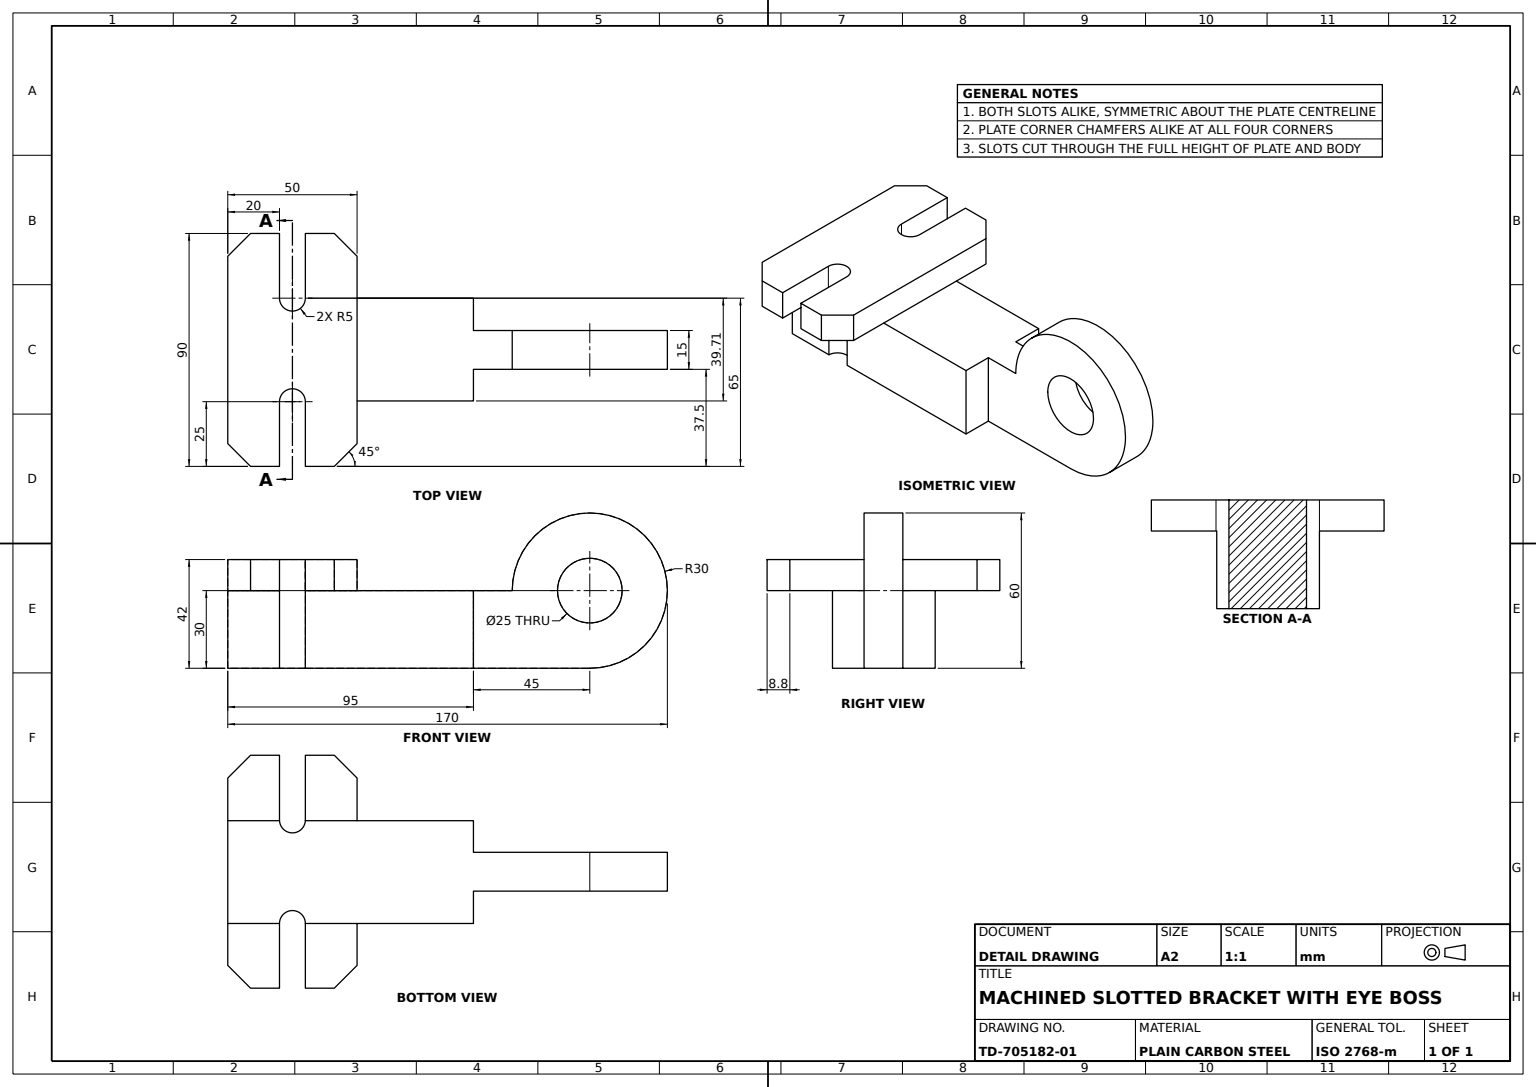
from build123d import *

# Parameters (mm, degrees)
BASE_BODY_42MM_DEPTH = 42
SKETCH1_5_W          = 15
SKETCH1_5_H          = 15
SIDE_BOSS_30MM_DEPTH = 30
SLOTS_SKETCH_W       = 16.483923251
SLOTS_SKETCH_H       = 30
SLOTS_SKETCH_W_2     = 8.802682669
SLOTS_SKETCH_W_3     = 16.197317331
SLOTS_CUT_DEPTH      = 123
SKETCH1_6_W          = 30
SKETCH1_6_H          = 15
EYE_BOSS_70MM_DEPTH  = 70
WEB_SKETCH_W         = 30
WEB_SKETCH_H         = 15
WEB_BOSS_70MM_DEPTH  = 70
PIN_BORE_SKETCH_R    = 12.5
PIN_BORE_CUT_DEPTH   = 15


with BuildPart() as part:
    # Link Profile Sketch → Base Body 42mm (new body)
    with BuildSketch(Plane(origin=(0, 0, 0), x_dir=(1, 0, 0), z_dir=(0, 1, 0))):
        with BuildLine():
            Line((20, -20), (20, -45))
            Line((20, -45), (8.802682669, -45))
            Line((8.802682669, -45), (0, -36.197317331))
            Line((0, -36.197317331), (0, 0))
            Line((0, 0), (0, 36.197317331))
            Line((0, 36.197317331), (8.802682669, 45))
            Line((8.802682669, 45), (20, 45))
            Line((20, 45), (20, 20))
            ThreePointArc((20, 20), (25, 15), (30, 20))
            Line((30, 20), (30, 45))
            Line((30, 45), (41.197317331, 45))
            Line((41.197317331, 45), (50, 36.197317331))
            Line((50, 36.197317331), (50, -36.197317331))
            Line((50, -36.197317331), (41.197317331, -45))
            Line((41.197317331, -45), (30, -45))
            Line((30, -45), (30, -20))
            ThreePointArc((30, -20), (25, -15), (20, -20))
        make_face()
    extrude(amount=BASE_BODY_42MM_DEPTH)

    # Sketch1_5 → Side Boss 30mm (add)
    with BuildSketch(Plane(origin=(0, 0, 0), x_dir=(1, 0, 0), z_dir=(0, 1, 0))):
        Polygon((95, 20), (50, 20), (50, -20), (95, -20), (95, -7.5), (95, 7.5), align=None)
        with Locations((102.5, 0)):
            Rectangle(SKETCH1_5_W, SKETCH1_5_H)
    extrude(amount=SIDE_BOSS_30MM_DEPTH)

    # Slots Sketch → Slots Cut (cut)
    with BuildSketch(Plane.ZY):
        with Locations((27.955355706, 15)):
            Rectangle(SLOTS_SKETCH_W, SLOTS_SKETCH_H)
        with Locations((40.598658665, 15)):
            Rectangle(SLOTS_SKETCH_W_2, SLOTS_SKETCH_H)
        with Locations((-28.098658666, 15)):
            Rectangle(SLOTS_SKETCH_W_3, SLOTS_SKETCH_H)
        with Locations((-40.598658665, 15)):
            Rectangle(SLOTS_SKETCH_W_2, SLOTS_SKETCH_H)
    extrude(amount=-SLOTS_CUT_DEPTH, mode=Mode.SUBTRACT)

    # Sketch1_6 → Eye Boss 70mm (add)
    with BuildSketch(Plane(origin=(0, 0, 0), x_dir=(1, 0, 0), z_dir=(0, 1, 0))):
        with Locations((125, 0)):
            Rectangle(SKETCH1_6_W, SKETCH1_6_H)
    extrude(amount=EYE_BOSS_70MM_DEPTH)

    # Web Sketch → Web Boss 70mm (add)
    with BuildSketch(Plane(origin=(0, 70, 0), x_dir=(1, 0, 0), z_dir=(0, 1, 0))):
        with Locations((155, 0)):
            Rectangle(WEB_SKETCH_W, WEB_SKETCH_H)
    extrude(amount=-WEB_BOSS_70MM_DEPTH)

    # Pin Bore Sketch → Pin Bore Cut (cut)
    with BuildSketch(Plane.XY.offset(7.5)):
        with Locations((140, 30)):
            Circle(PIN_BORE_SKETCH_R)
        with BuildLine():
            Line((110, 70), (110, 30))
            ThreePointArc((110, 30), (140, 60), (170, 30))
            Line((170, 30), (170, 70))
            Line((170, 70), (110, 70))
        make_face()
        with BuildLine():
            Line((170, 0), (170, 30))
            ThreePointArc((170, 30), (161.213203436, 8.786796564), (140, 0))
            Line((140, 0), (170, 0))
        make_face()
    extrude(amount=-PIN_BORE_CUT_DEPTH, mode=Mode.SUBTRACT)


solid = part.part
